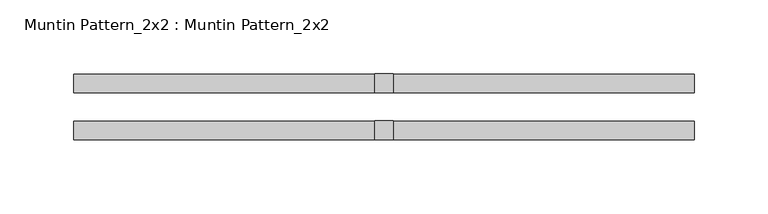
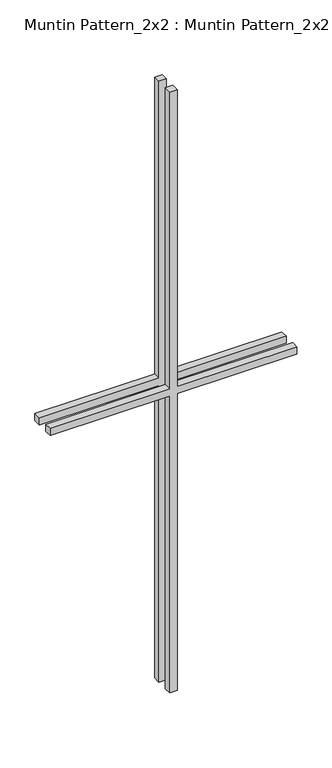
"""IFC4 building model written with IfcOpenShell, lengths in millimetres: proxy geometry, Muntin Pattern_2x2 : Muntin Pattern_2x2."""

from ifc_helpers import new_model, si_unit, frame, origin, place, context, project, spatial, polyline, outline, extrude, source, transform, mapped, element, save


def muntin_pattern_2x2_muntin_pattern_2x2_eb08c668(model_context):
    return source(origin(), model_context, "Body", "SweptSolid", [
        extrude(outline(polyline([(546.1, -6.35), (546.1, -209.55), (533.4, -209.55), (533.4, -6.35), (0.0, -6.35), (0.0, 6.35), (533.4, 6.35), (533.4, 209.55), (546.1, 209.55), (546.1, 6.35), (1079.5, 6.35), (1079.5, -6.35), (546.1, -6.35)])), frame((0.0, -22.225, 0.0), z_axis=(0.0, 1.0, 0.0), x_axis=(0.0, 0.0, 1.0)), (0.0, 0.0, 1.0), 12.7),
        extrude(outline(polyline([(546.1, -6.35), (546.1, -209.55), (533.4, -209.55), (533.4, -6.35), (0.0, -6.35), (0.0, 6.35), (533.4, 6.35), (533.4, 209.55), (546.1, 209.55), (546.1, 6.35), (1079.5, 6.35), (1079.5, -6.35), (546.1, -6.35)])), frame((0.0, 9.525, 0.0), z_axis=(0.0, 1.0, 0.0), x_axis=(0.0, 0.0, 1.0)), (0.0, 0.0, 1.0), 12.7),
    ])


if __name__ == "__main__":
    model = new_model("IFC4")
    model_context = context("Model", 3, world=origin())
    ifc_project = project(units=[si_unit("LENGTHUNIT", "METRE", prefix="MILLI")], contexts=[model_context])
    site = spatial("IfcSite", under=ifc_project)
    building = spatial("IfcBuilding", under=site)
    placement = place(None, origin())
    muntin_pattern_2x2_muntin_pattern_2x2_shape = muntin_pattern_2x2_muntin_pattern_2x2_eb08c668(model_context)
    element("IfcBuildingElementProxy", 1, Name="Muntin Pattern_2x2 : Muntin Pattern_2x2", ObjectType="Muntin Pattern_2x2 : Muntin Pattern_2x2", at=placement, inside=building, context=model_context, shape_type="MappedRepresentation", body=[
        mapped(muntin_pattern_2x2_muntin_pattern_2x2_shape, transform((0.0, 0.0, 0.0), x_axis=(1.0, 0.0, 0.0), y_axis=(0.0, 1.0, 0.0), z_axis=(0.0, 0.0, 1.0))),
    ])
    save(model, "model.ifc")

# Revit data of these elements
# Type "Muntin Pattern_2x2 : Muntin Pattern_2x2"
#   Width [instance default] = 4' - 0"
#   Thickness = 0' - 0 1/2"
#   Height [instance default] = 4' - 0"
#   Distance = 0' - 0 3/4"
#   Interior Material [instance default] = none
#   Exterior Material [instance default] = none
#   Default Elevation = 0
# Element 1 (IfcBuildingElementProxy, "Muntin Pattern_2x2 : Muntin Pattern_2x2")
#   Width = 1' - 4 1/2"
#   Height = 3' - 6 1/2"
#   Interior Material = Wood - Stained
#   Exterior Material = Clad - White
#   Materials on its faces: "Clad - White", "Wood - Stained"
# Materials
#   "Clad - White": class "Wood", colour RGB 242 242 238, transparency 0, Cost = 0
#   "Wood - Stained": class "Wood", colour RGB 224 178 126, transparency 0, Cost = 0
